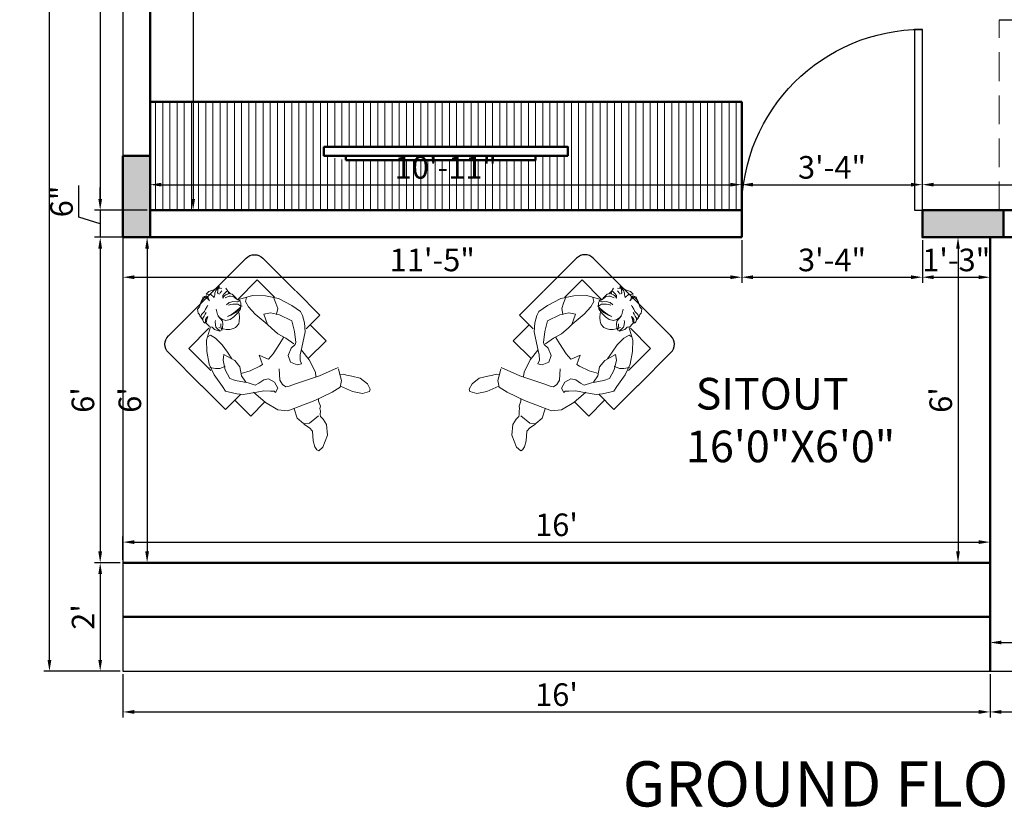
# Model space of a CAD drawing. Units: inches. Extents: x 3064 to 19385, y 846 to 15425.
# Tile 81 of 108: x 7077 to 7295, y 850 to 1024. Entities that reach past the tile are written whole.
import ezdxf

# ---------------------------------------------------------------- set-up
doc = ezdxf.new("R2010")
doc.units = ezdxf.units.IN
doc.linetypes.add('DASHED', pattern=[19.05, 12.7, -6.35])
for name, color, linetype, lineweight in [('A-ANNO-DIMS', 2, 'Continuous', 18), ('A-ANNO-TEXT', 7, 'Continuous', 25), ('A-AREA-IDEN', 3, 'Continuous', 18), ('A-COLS', 1, 'Continuous', 35), ('A-DOOR', 3, 'Continuous', 25), ('A-FLOR-STRS', 2, 'Continuous', 25), ('A-FLOR-STRS-OVHD', 2, 'DASHED', 18), ('A-FURN', 8, 'Continuous', 18), ('A-FURN-PATT', 252, 'Continuous', 13), ('A-WALL', 7, 'Continuous', 50), ('C-PROP', 6, 'Continuous', 25)]:
    doc.layers.add(name, color=color, linetype=linetype, lineweight=lineweight)
doc.layers.add('NOITHAT', color=21, linetype='Continuous')
doc.styles.get("Standard").update_dxf_attribs({"font": 'arial.ttf'})
doc.dimstyles.new('ISO-25', dxfattribs={"dimtxt": 9, "dimasz": 2.5, "dimexe": 1.25, "dimexo": 0.625, "dimtad": 1, "dimdec": 1, "dimlunit": 3, "dimtxsty": 'Standard', "dimcen": 2.5, "dimadec": 0, "dimazin": 0, "dimtfac": 1, "dimtdec": 1, "dimtmove": 0, "dimatfit": 3, "dimfxl": 1, "dimarcsym": 0})

# ---------------------------------------------------------------- blocks, each defined once
blk = doc.blocks.new('*U2')
for p, q in [((0, 0), (0, -6)), ((40, 0), (40, -6))]:
    blk.add_line(p, q)
blk.add_lwpolyline([(0, 0), (0, 40), (1.75, 40), (1.75, 0)], close=True)
blk.add_arc((0, 0), 40, 0, 90)
blk = doc.blocks.new('*D299')
at = {"layer": 'A-ANNO-DIMS', "color": 0, "lineweight": -2, "transparency": 16777216}
for p, q in [((7099.08, 1252.34), (7093.43, 1252.34)), ((7094.68, 1249.84), (7094.68, 984.84)), ((7105.08, 982.34), (7093.43, 982.34))]:
    blk.add_line(p, q, dxfattribs=at)
at = {"layer": 'A-ANNO-DIMS', "color": 0, "transparency": 16777216}
for points in [[(7094.26, 1249.84), (7095.09, 1249.84), (7094.68, 1252.34)], [(7094.26, 984.84), (7095.09, 984.84), (7094.68, 982.34)]]:
    blk.add_solid(points, dxfattribs=at)
at = {"layer": 'Defpoints', "color": 0, "transparency": 16777216}
for p in [(7099.71, 1252.34), (7094.68, 982.34), (7105.71, 982.34)]:
    blk.add_point(p, dxfattribs=at)
at = {"layer": 'A-ANNO-DIMS', "color": 0, "transparency": 16777216, "insert": (7091.5, 1117.34), "char_height": 5, "attachment_point": 5, "rotation": 90}
blk.add_mtext('22\'-6"', dxfattribs=at)
blk = doc.blocks.new('*D300')
at = {"layer": 'A-ANNO-DIMS', "color": 0, "lineweight": -2, "transparency": 16777216}
for p, q in [((7089.94, 980.76), (7089.94, 987.79)), ((7094.68, 984.84), (7094.68, 987.34)), ((7105.08, 982.34), (7093.43, 982.34)), ((7094.68, 982.34), (7094.68, 976.34)), ((7094.68, 982.34), (7094.68, 976.34)), ((7094.68, 979.34), (7089.94, 980.76)), ((7105.08, 976.34), (7093.43, 976.34)), ((7094.68, 973.84), (7094.68, 971.34))]:
    blk.add_line(p, q, dxfattribs=at)
at = {"layer": 'A-ANNO-DIMS', "color": 0, "transparency": 16777216}
for points in [[(7094.26, 984.84), (7095.09, 984.84), (7094.68, 982.34)], [(7094.26, 973.84), (7095.09, 973.84), (7094.68, 976.34)]]:
    blk.add_solid(points, dxfattribs=at)
at = {"layer": 'Defpoints', "color": 0, "transparency": 16777216}
for p in [(7105.71, 982.34), (7094.68, 976.34), (7105.71, 976.34)]:
    blk.add_point(p, dxfattribs=at)
at = {"layer": 'A-ANNO-DIMS', "color": 0, "transparency": 16777216, "insert": (7086.76, 984.27), "char_height": 5, "attachment_point": 5, "rotation": 90}
blk.add_mtext('6"', dxfattribs=at)
blk = doc.blocks.new('*D301')
at = {"layer": 'A-ANNO-DIMS', "color": 0, "lineweight": -2, "transparency": 16777216}
for p, q in [((7105.08, 976.34), (7093.43, 976.34)), ((7094.68, 973.84), (7094.68, 906.84)), ((7099.08, 904.34), (7093.43, 904.34))]:
    blk.add_line(p, q, dxfattribs=at)
at = {"layer": 'A-ANNO-DIMS', "color": 0, "transparency": 16777216}
for points in [[(7094.26, 973.84), (7095.09, 973.84), (7094.68, 976.34)], [(7094.26, 906.84), (7095.09, 906.84), (7094.68, 904.34)]]:
    blk.add_solid(points, dxfattribs=at)
at = {"layer": 'Defpoints', "color": 0, "transparency": 16777216}
for p in [(7105.71, 976.34), (7094.68, 904.34), (7099.71, 904.34)]:
    blk.add_point(p, dxfattribs=at)
at = {"layer": 'A-ANNO-DIMS', "color": 0, "transparency": 16777216, "insert": (7091.5, 940.34), "char_height": 5, "attachment_point": 5, "rotation": 90}
blk.add_mtext("6'", dxfattribs=at)
blk = doc.blocks.new('*D302')
at = {"layer": 'A-ANNO-DIMS', "color": 0, "lineweight": -2, "transparency": 16777216}
for p, q in [((7099.08, 904.34), (7093.43, 904.34)), ((7094.68, 901.84), (7094.68, 882.84)), ((7099.08, 880.34), (7093.43, 880.34))]:
    blk.add_line(p, q, dxfattribs=at)
at = {"layer": 'A-ANNO-DIMS', "color": 0, "transparency": 16777216}
for points in [[(7094.26, 901.84), (7095.09, 901.84), (7094.68, 904.34)], [(7094.26, 882.84), (7095.09, 882.84), (7094.68, 880.34)]]:
    blk.add_solid(points, dxfattribs=at)
at = {"layer": 'Defpoints', "color": 0, "transparency": 16777216}
for p in [(7099.71, 904.34), (7094.68, 880.34), (7099.71, 880.34)]:
    blk.add_point(p, dxfattribs=at)
at = {"layer": 'A-ANNO-DIMS', "color": 0, "transparency": 16777216, "insert": (7091.54, 892.34), "char_height": 5, "attachment_point": 5, "rotation": 90}
blk.add_mtext("2'", dxfattribs=at)
blk = doc.blocks.new('*D303')
at = {"layer": 'A-ANNO-DIMS', "color": 0, "lineweight": -2, "transparency": 16777216}
for p, q in [((7099.08, 1396.34), (7082.19, 1396.34)), ((7083.44, 882.84), (7083.44, 1393.84)), ((7099.08, 880.34), (7082.19, 880.34))]:
    blk.add_line(p, q, dxfattribs=at)
at = {"layer": 'A-ANNO-DIMS', "color": 0, "transparency": 16777216}
for points in [[(7083.02, 1393.84), (7083.86, 1393.84), (7083.44, 1396.34)], [(7083.02, 882.84), (7083.86, 882.84), (7083.44, 880.34)]]:
    blk.add_solid(points, dxfattribs=at)
at = {"layer": 'Defpoints', "color": 0, "transparency": 16777216}
for p in [(7083.44, 1396.34), (7099.71, 1396.34), (7099.71, 880.34)]:
    blk.add_point(p, dxfattribs=at)
at = {"layer": 'A-ANNO-DIMS', "color": 0, "transparency": 16777216, "insert": (7080.26, 1138.34), "char_height": 5, "attachment_point": 5, "rotation": 90}
blk.add_mtext("43'", dxfattribs=at)
blk = doc.blocks.new('*D304')
at = {"layer": 'A-ANNO-DIMS', "color": 0, "lineweight": -2, "transparency": 16777216}
for p, q in [((7099.71, 879.71), (7099.71, 870.08)), ((7291.71, 879.71), (7291.71, 870.08)), ((7102.21, 871.33), (7289.21, 871.33))]:
    blk.add_line(p, q, dxfattribs=at)
at = {"layer": 'A-ANNO-DIMS', "color": 0, "transparency": 16777216}
for points in [[(7102.21, 871.75), (7102.21, 870.91), (7099.71, 871.33)], [(7289.21, 871.75), (7289.21, 870.91), (7291.71, 871.33)]]:
    blk.add_solid(points, dxfattribs=at)
at = {"layer": 'Defpoints', "color": 0, "transparency": 16777216}
for p in [(7099.71, 880.34), (7291.71, 880.34), (7291.71, 871.33)]:
    blk.add_point(p, dxfattribs=at)
at = {"layer": 'A-ANNO-DIMS', "color": 0, "transparency": 16777216, "insert": (7195.71, 874.51), "char_height": 5, "attachment_point": 5}
blk.add_mtext("16'", dxfattribs=at)
blk = doc.blocks.new('*D305')
at = {"layer": 'A-ANNO-DIMS', "color": 0, "lineweight": -2, "transparency": 16777216}
for p, q in [((7291.71, 879.71), (7291.71, 870.08)), ((7441.71, 879.71), (7441.71, 870.08)), ((7294.21, 871.33), (7439.21, 871.33))]:
    blk.add_line(p, q, dxfattribs=at)
at = {"layer": 'A-ANNO-DIMS', "color": 0, "transparency": 16777216}
for points in [[(7294.21, 871.75), (7294.21, 870.91), (7291.71, 871.33)], [(7439.21, 871.75), (7439.21, 870.91), (7441.71, 871.33)]]:
    blk.add_solid(points, dxfattribs=at)
at = {"layer": 'Defpoints', "color": 0, "transparency": 16777216}
for p in [(7291.71, 880.34), (7441.71, 880.34), (7441.71, 871.33)]:
    blk.add_point(p, dxfattribs=at)
at = {"layer": 'A-ANNO-DIMS', "color": 0, "transparency": 16777216, "insert": (7366.71, 874.51), "char_height": 5, "attachment_point": 5}
blk.add_mtext('12\'-6"', dxfattribs=at)
blk = doc.blocks.new('*D223')
at = {"layer": 'A-ANNO-DIMS', "color": 0, "lineweight": -2, "transparency": 16777216}
for p, q in [((7106.33, 1252.34), (7116.51, 1252.34)), ((7115.26, 1249.84), (7115.26, 984.84)), ((7106.33, 982.34), (7116.51, 982.34))]:
    blk.add_line(p, q, dxfattribs=at)
at = {"layer": 'A-ANNO-DIMS', "color": 0, "transparency": 16777216}
for points in [[(7114.84, 1249.84), (7115.67, 1249.84), (7115.26, 1252.34)], [(7114.84, 984.84), (7115.67, 984.84), (7115.26, 982.34)]]:
    blk.add_solid(points, dxfattribs=at)
at = {"layer": 'Defpoints', "color": 0, "transparency": 16777216}
for p in [(7105.71, 1252.34), (7105.71, 982.34), (7115.26, 982.34)]:
    blk.add_point(p, dxfattribs=at)
at = {"layer": 'A-ANNO-DIMS', "color": 0, "transparency": 16777216, "insert": (7112.08, 1117.34), "char_height": 5, "attachment_point": 5, "rotation": 90}
blk.add_mtext('22\'-6"', dxfattribs=at)
blk = doc.blocks.new('*D272')
at = {"layer": 'A-ANNO-DIMS', "color": 0, "lineweight": -2, "transparency": 16777216}
for p, q in [((7105.71, 982.96), (7105.71, 989.23)), ((7108.21, 987.98), (7234.21, 987.98)), ((7236.71, 982.96), (7236.71, 989.23))]:
    blk.add_line(p, q, dxfattribs=at)
at = {"layer": 'A-ANNO-DIMS', "color": 0, "transparency": 16777216}
for points in [[(7108.21, 988.4), (7108.21, 987.57), (7105.71, 987.98)], [(7234.21, 988.4), (7234.21, 987.57), (7236.71, 987.98)]]:
    blk.add_solid(points, dxfattribs=at)
at = {"layer": 'Defpoints', "color": 0, "transparency": 16777216}
for p in [(7236.71, 987.98), (7105.71, 982.34), (7236.71, 982.34)]:
    blk.add_point(p, dxfattribs=at)
at = {"layer": 'A-ANNO-DIMS', "color": 0, "transparency": 16777216, "insert": (7171.21, 991.16), "char_height": 5, "attachment_point": 5}
blk.add_mtext('10\'-11"', dxfattribs=at)
blk = doc.blocks.new('*D273')
at = {"layer": 'A-ANNO-DIMS', "color": 0, "lineweight": -2, "transparency": 16777216}
for p, q in [((7236.71, 982.96), (7236.71, 989.23)), ((7239.21, 987.98), (7274.21, 987.98)), ((7276.71, 982.96), (7276.71, 989.23))]:
    blk.add_line(p, q, dxfattribs=at)
at = {"layer": 'A-ANNO-DIMS', "color": 0, "transparency": 16777216}
for points in [[(7239.21, 988.4), (7239.21, 987.57), (7236.71, 987.98)], [(7274.21, 988.4), (7274.21, 987.57), (7276.71, 987.98)]]:
    blk.add_solid(points, dxfattribs=at)
at = {"layer": 'Defpoints', "color": 0, "transparency": 16777216}
for p in [(7276.71, 987.98), (7236.71, 982.34), (7276.71, 982.34)]:
    blk.add_point(p, dxfattribs=at)
at = {"layer": 'A-ANNO-DIMS', "color": 0, "transparency": 16777216, "insert": (7256.71, 991.16), "char_height": 5, "attachment_point": 5}
blk.add_mtext('3\'-4"', dxfattribs=at)
blk = doc.blocks.new('*D274')
at = {"layer": 'A-ANNO-DIMS', "color": 0, "lineweight": -2, "transparency": 16777216}
for p, q in [((7276.71, 982.96), (7276.71, 989.23)), ((7279.21, 987.98), (7433.21, 987.98)), ((7435.71, 982.96), (7435.71, 989.23))]:
    blk.add_line(p, q, dxfattribs=at)
at = {"layer": 'A-ANNO-DIMS', "color": 0, "transparency": 16777216}
for points in [[(7279.21, 988.4), (7279.21, 987.57), (7276.71, 987.98)], [(7433.21, 988.4), (7433.21, 987.57), (7435.71, 987.98)]]:
    blk.add_solid(points, dxfattribs=at)
at = {"layer": 'Defpoints', "color": 0, "transparency": 16777216}
for p in [(7435.71, 987.98), (7276.71, 982.34), (7435.71, 982.34)]:
    blk.add_point(p, dxfattribs=at)
at = {"layer": 'A-ANNO-DIMS', "color": 0, "transparency": 16777216, "insert": (7356.21, 991.16), "char_height": 5, "attachment_point": 5}
blk.add_mtext('13\'-3"', dxfattribs=at)
blk = doc.blocks.new('*D240')
at = {"layer": 'A-ANNO-DIMS', "color": 0, "lineweight": -2, "transparency": 16777216}
for p, q in [((7100.33, 976.34), (7106.32, 976.34)), ((7105.07, 973.84), (7105.07, 906.84)), ((7100.33, 904.34), (7106.32, 904.34))]:
    blk.add_line(p, q, dxfattribs=at)
at = {"layer": 'A-ANNO-DIMS', "color": 0, "transparency": 16777216}
for points in [[(7104.65, 973.84), (7105.48, 973.84), (7105.07, 976.34)], [(7104.65, 906.84), (7105.48, 906.84), (7105.07, 904.34)]]:
    blk.add_solid(points, dxfattribs=at)
at = {"layer": 'Defpoints', "color": 0, "transparency": 16777216}
for p in [(7099.71, 976.34), (7099.71, 904.34), (7105.07, 904.34)]:
    blk.add_point(p, dxfattribs=at)
at = {"layer": 'A-ANNO-DIMS', "color": 0, "transparency": 16777216, "insert": (7101.89, 940.34), "char_height": 5, "attachment_point": 5, "rotation": 90}
blk.add_mtext("6'", dxfattribs=at)
blk = doc.blocks.new('*D241')
at = {"layer": 'A-ANNO-DIMS', "color": 0, "lineweight": -2, "transparency": 16777216}
for p, q in [((7099.71, 975.71), (7099.71, 966.25)), ((7236.71, 975.71), (7236.71, 966.25)), ((7102.21, 967.5), (7234.21, 967.5))]:
    blk.add_line(p, q, dxfattribs=at)
at = {"layer": 'A-ANNO-DIMS', "color": 0, "transparency": 16777216}
for points in [[(7102.21, 967.92), (7102.21, 967.09), (7099.71, 967.5)], [(7234.21, 967.92), (7234.21, 967.09), (7236.71, 967.5)]]:
    blk.add_solid(points, dxfattribs=at)
at = {"layer": 'Defpoints', "color": 0, "transparency": 16777216}
for p in [(7099.71, 976.34), (7236.71, 976.34), (7236.71, 967.5)]:
    blk.add_point(p, dxfattribs=at)
at = {"layer": 'A-ANNO-DIMS', "color": 0, "transparency": 16777216, "insert": (7168.21, 970.68), "char_height": 5, "attachment_point": 5}
blk.add_mtext('11\'-5"', dxfattribs=at)
blk = doc.blocks.new('*D267')
at = {"layer": 'A-ANNO-DIMS', "color": 0, "lineweight": -2, "transparency": 16777216}
for p, q in [((7236.71, 975.71), (7236.71, 966.25)), ((7276.71, 975.71), (7276.71, 966.25)), ((7239.21, 967.5), (7274.21, 967.5))]:
    blk.add_line(p, q, dxfattribs=at)
at = {"layer": 'A-ANNO-DIMS', "color": 0, "transparency": 16777216}
for points in [[(7239.21, 967.92), (7239.21, 967.09), (7236.71, 967.5)], [(7274.21, 967.92), (7274.21, 967.09), (7276.71, 967.5)]]:
    blk.add_solid(points, dxfattribs=at)
at = {"layer": 'Defpoints', "color": 0, "transparency": 16777216}
for p in [(7236.71, 976.34), (7276.71, 976.34), (7276.71, 967.5)]:
    blk.add_point(p, dxfattribs=at)
at = {"layer": 'A-ANNO-DIMS', "color": 0, "transparency": 16777216, "insert": (7256.71, 970.68), "char_height": 5, "attachment_point": 5}
blk.add_mtext('3\'-4"', dxfattribs=at)
blk = doc.blocks.new('*D268')
at = {"layer": 'A-ANNO-DIMS', "color": 0, "lineweight": -2, "transparency": 16777216}
for p, q in [((7276.71, 975.71), (7276.71, 966.25)), ((7291.71, 975.71), (7291.71, 966.25)), ((7279.21, 967.5), (7289.21, 967.5))]:
    blk.add_line(p, q, dxfattribs=at)
at = {"layer": 'A-ANNO-DIMS', "color": 0, "transparency": 16777216}
for points in [[(7279.21, 967.92), (7279.21, 967.09), (7276.71, 967.5)], [(7289.21, 967.92), (7289.21, 967.09), (7291.71, 967.5)]]:
    blk.add_solid(points, dxfattribs=at)
at = {"layer": 'Defpoints', "color": 0, "transparency": 16777216}
for p in [(7276.71, 976.34), (7291.71, 976.34), (7291.71, 967.5)]:
    blk.add_point(p, dxfattribs=at)
at = {"layer": 'A-ANNO-DIMS', "color": 0, "transparency": 16777216, "insert": (7284.21, 970.68), "char_height": 5, "attachment_point": 5}
blk.add_mtext('1\'-3"', dxfattribs=at)
blk = doc.blocks.new('*D269')
at = {"layer": 'A-ANNO-DIMS', "color": 0, "lineweight": -2, "transparency": 16777216}
for p, q in [((7099.71, 904.96), (7099.71, 910.15)), ((7291.71, 904.96), (7291.71, 910.15)), ((7102.21, 908.9), (7289.21, 908.9))]:
    blk.add_line(p, q, dxfattribs=at)
at = {"layer": 'A-ANNO-DIMS', "color": 0, "transparency": 16777216}
for points in [[(7102.21, 909.32), (7102.21, 908.49), (7099.71, 908.9)], [(7289.21, 909.32), (7289.21, 908.49), (7291.71, 908.9)]]:
    blk.add_solid(points, dxfattribs=at)
at = {"layer": 'Defpoints', "color": 0, "transparency": 16777216}
for p in [(7291.71, 908.9), (7099.71, 904.34), (7291.71, 904.34)]:
    blk.add_point(p, dxfattribs=at)
at = {"layer": 'A-ANNO-DIMS', "color": 0, "transparency": 16777216, "insert": (7195.71, 912.08), "char_height": 5, "attachment_point": 5}
blk.add_mtext("16'", dxfattribs=at)
blk = doc.blocks.new('*D270')
at = {"layer": 'A-ANNO-DIMS', "color": 0, "lineweight": -2, "transparency": 16777216}
for p, q in [((7291.08, 976.34), (7283.35, 976.34)), ((7284.6, 973.84), (7284.6, 906.84)), ((7291.08, 904.34), (7283.35, 904.34))]:
    blk.add_line(p, q, dxfattribs=at)
at = {"layer": 'A-ANNO-DIMS', "color": 0, "transparency": 16777216}
for points in [[(7284.19, 973.84), (7285.02, 973.84), (7284.6, 976.34)], [(7284.19, 906.84), (7285.02, 906.84), (7284.6, 904.34)]]:
    blk.add_solid(points, dxfattribs=at)
at = {"layer": 'Defpoints', "color": 0, "transparency": 16777216}
for p in [(7291.71, 976.34), (7284.6, 904.34), (7291.71, 904.34)]:
    blk.add_point(p, dxfattribs=at)
at = {"layer": 'A-ANNO-DIMS', "color": 0, "transparency": 16777216, "insert": (7281.43, 940.34), "char_height": 5, "attachment_point": 5, "rotation": 90}
blk.add_mtext("6'", dxfattribs=at)
blk = doc.blocks.new('*D221')
at = {"layer": 'A-ANNO-DIMS', "color": 0, "lineweight": -2, "transparency": 16777216}
for p, q in [((7291.71, 880.96), (7291.71, 887.94)), ((7441.71, 880.96), (7441.71, 887.94)), ((7294.21, 886.69), (7439.21, 886.69))]:
    blk.add_line(p, q, dxfattribs=at)
at = {"layer": 'A-ANNO-DIMS', "color": 0, "transparency": 16777216}
for points in [[(7294.21, 887.11), (7294.21, 886.28), (7291.71, 886.69)], [(7439.21, 887.11), (7439.21, 886.28), (7441.71, 886.69)]]:
    blk.add_solid(points, dxfattribs=at)
at = {"layer": 'Defpoints', "color": 0, "transparency": 16777216}
for p in [(7441.71, 886.69), (7291.71, 880.34), (7441.71, 880.34)]:
    blk.add_point(p, dxfattribs=at)
at = {"layer": 'A-ANNO-DIMS', "color": 0, "transparency": 16777216, "insert": (7366.71, 889.87), "char_height": 5, "attachment_point": 5}
blk.add_mtext('12\'-6"', dxfattribs=at)
blk = doc.blocks.new('A$C48E80792')
for p, q in [((230.8, 792.5), (252, 804.1)), ((252, 804.1), (267.8, 807.6)), ((253.5, 801.9), (261.1, 805.7)), ((261.1, 805.7), (274.4, 805.7)), ((267.8, 807.6), (270.5, 811.7)), ((284, 805.7), (270.6, 811.4)), ((274.4, 805.7), (278.3, 805.7)), ((278.3, 805.7), (278.3, 798.1)), ((278.3, 798.1), (280.2, 788.5)), ((284, 794.3), (284, 805.7)), ((289.7, 811.4), (305.5, 811.7)), ((289.7, 811.4), (303, 796.2)), ((305.5, 811.7), (317.9, 805.5)), ((317.9, 805.5), (328.1, 800)), ((328.1, 800), (343.9, 798)), ((343.9, 798), (352.1, 795.9)), ((202, 746.6), (204.7, 764.4)), ((202, 746.6), (205.8, 759.9)), ((204.7, 764.4), (207.4, 769.9)), ((205.8, 759.9), (213.4, 763.8)), ((207.4, 769.9), (208.1, 777.4)), ((208.1, 777.4), (217.7, 791.8)), ((213.4, 763.8), (222.9, 763.8)), ((217.7, 791.8), (230.8, 792.5)), ((222.9, 763.8), (232.5, 763.8)), ((226.8, 754.2), (234.4, 756.1)), ((232.5, 763.8), (236.3, 765.7)), ((236.3, 765.7), (242, 767.6)), ((242, 767.6), (255.4, 771.4)), ((255.4, 771.4), (261.1, 773.3)), ((280.2, 786.6), (284, 794.3)), ((280.2, 788.5), (280.2, 780.9)), ((280.2, 780.9), (280.2, 786.6)), ((303, 796.2), (303, 779)), ((303, 777.1), (312.6, 782.8)), ((303, 779), (303, 777.1)), ((312.6, 782.8), (318.3, 788.5)), ((318.3, 788.5), (329.8, 792.4)), ((335.5, 786.6), (327.8, 780.9)), ((327.8, 780.9), (327.8, 775.2)), ((327.8, 748.5), (335.5, 756.1)), ((329.8, 792.4), (343.1, 794.3)), ((329.8, 771.4), (335.5, 773.3)), ((343.1, 792.4), (335.5, 786.6)), ((335.5, 773.3), (346.9, 773.3)), ((335.5, 756.1), (346.9, 758)), ((343.1, 794.3), (352.6, 794.3)), ((352.6, 792.4), (343.1, 792.4)), ((343.9, 790.4), (354.9, 782.2)), ((346.9, 758), (358.4, 758)), ((358.4, 758), (362.2, 756.1)), ((366, 769.5), (362.2, 750.4)), ((362.2, 756.1), (364.1, 750.4)), ((198.1, 735.2), (202, 742.8)), ((198.1, 727.5), (198.1, 735.2)), ((202, 727.5), (200.1, 725.6)), ((202, 742.8), (207.7, 748.5)), ((211.5, 737.1), (202, 727.5)), ((202, 723.7), (209.6, 729.4)), ((202, 716.1), (202, 723.7)), ((202, 706.6), (202, 716.1)), ((207.7, 748.5), (217.2, 750.4)), ((209.6, 729.4), (219.1, 735.2)), ((219.1, 739), (211.5, 737.1)), ((217.2, 750.4), (226.8, 754.2)), ((226.8, 739), (219.1, 739)), ((219.1, 735.2), (226.8, 739)), ((226.8, 739), (226.8, 739)), ((261.6, 715.7), (260.3, 708.9)), ((274, 735.6), (261.6, 715.7)), ((318.3, 718), (333.6, 716.1)), ((329.8, 748.5), (327.8, 748.5)), ((335.5, 750.4), (329.8, 748.5)), ((333.6, 716.1), (339.3, 712.3)), ((337.4, 750.4), (335.5, 750.4)), ((352.6, 735.2), (335.5, 742.8)), ((341.2, 750.4), (337.4, 750.4)), ((346.9, 750.4), (341.2, 750.4)), ((354.5, 746.6), (346.9, 750.4)), ((356.5, 731.3), (352.6, 735.2)), ((362.2, 742.8), (354.5, 746.6)), ((362.2, 750.4), (356.5, 746.6)), ((362.2, 723.7), (356.5, 731.3)), ((367.9, 733.3), (362.2, 742.8)), ((364.1, 718), (362.2, 723.7)), ((364.1, 750.4), (364.1, 742.8)), ((364.1, 742.8), (364.1, 739)), ((366, 706.6), (364.1, 718)), ((367.9, 706.6), (367.9, 733.3)), ((151.7, 671.2), (119.2, 637.1)), ((204, 699.4), (151.7, 671.2)), ((165.1, 679.5), (178.4, 675)), ((178.4, 675), (185.1, 650.5)), ((202, 702.8), (202, 706.6)), ((207.7, 693.2), (202, 702.8)), ((207.7, 679.9), (207.7, 693.2)), ((219.1, 658.9), (207.7, 679.9)), ((219.1, 681.8), (224.8, 691.3)), ((219.1, 670.3), (219.1, 681.8)), ((224.8, 691.3), (232.5, 700.8)), ((227.3, 673.2), (235.6, 655.4)), ((232.5, 700.8), (238.2, 704.7)), ((236.3, 670.3), (243.9, 678)), ((257.3, 679.9), (249.6, 670.3)), ((259.2, 708.5), (257.3, 679.9)), ((260.3, 708.9), (259.6, 699.3)), ((259.6, 699.3), (261.6, 685.6)), ((261.6, 685.6), (269.2, 671.8)), ((269.2, 671.8), (285.6, 662.9)), ((302.1, 672.5), (287, 679.4)), ((287, 679.4), (304.8, 673.9)), ((323.3, 667), (302.1, 672.5)), ((304.8, 673.9), (323.3, 670.5)), ((331.7, 706.6), (324, 710.4)), ((339.3, 700.8), (331.7, 706.6)), ((339.3, 712.3), (346.9, 708.5)), ((346.9, 693.2), (339.3, 700.8)), ((346.9, 708.5), (358.4, 695.1)), ((354.5, 685.6), (346.9, 693.2)), ((356.5, 676.1), (354.5, 685.6)), ((356.3, 668.4), (367.2, 680.1)), ((362.2, 666.5), (356.5, 676.1)), ((358.4, 695.1), (360.3, 693.2)), ((360.3, 693.2), (366, 691.3)), ((367.9, 698.9), (366, 706.6)), ((366, 691.3), (369.8, 689.4)), ((366.5, 698.9), (425.1, 668)), ((367.2, 680.1), (370.7, 689)), ((371.7, 691.3), (367.9, 698.9)), ((369.8, 689.4), (371.7, 689.4)), ((371.7, 689.4), (371.7, 691.3)), ((371.7, 689.4), (371.7, 689.4)), ((385.6, 670.5), (378.9, 646.1)), ((401.2, 679.5), (385.6, 670.5)), ((119.2, 637.1), (88.2, 591.5)), ((185.1, 650.5), (185.1, 610.4)), ((221, 657), (219.1, 670.3)), ((226.8, 655.1), (232.5, 664.6)), ((232.5, 657), (226.8, 655.1)), ((232.5, 664.6), (236.3, 670.3)), ((238.2, 660.8), (232.5, 657)), ((235.6, 655.4), (243.8, 644.4)), ((249.6, 670.3), (238.2, 660.8)), ((243.8, 644.4), (254.8, 633.5)), ((254.8, 633.5), (267.8, 625.9)), ((285.6, 662.9), (304.8, 659.5)), ((298, 623.9), (307.6, 630.7)), ((304.8, 659.5), (326.8, 659.5)), ((307.6, 630.7), (319.2, 640.3)), ((319.2, 640.3), (330.9, 654)), ((323.3, 670.5), (345.3, 668.4)), ((337.7, 666.4), (323.3, 667)), ((326.8, 659.5), (340.5, 661.6)), ((330.9, 654), (334, 660.6)), ((356.3, 669.8), (337.7, 666.4)), ((340.5, 661.6), (348.7, 664.3)), ((345.3, 668.4), (356.3, 668.4)), ((348.7, 664.3), (352.1, 667.7)), ((352.1, 667.7), (356.3, 669.8)), ((356.3, 668.4), (358.3, 669.8)), ((378.9, 646.1), (376.7, 603.8)), ((425.1, 668), (462.5, 627.3)), ((88.2, 591.5), (70.3, 544.3)), ((185.1, 610.4), (178.4, 572.6)), ((267.8, 625.9), (276.7, 622.5)), ((276.7, 622.5), (283.6, 621.8)), ((283.6, 621.8), (298, 623.9)), ((376.7, 603.8), (383.3, 537)), ((462.5, 627.3), (493.4, 580.1)), ((485.8, 606), (472.4, 574.8)), ((80.4, 579.3), (93.8, 559.2)), ((93.8, 559.2), (107.1, 545.9)), ((107.1, 545.9), (125, 539.2)), ((119.2, 526.5), (141.9, 562.2)), ((141.9, 562.2), (161.5, 576.9)), ((161.5, 576.9), (175.7, 525.7)), ((178.4, 572.6), (171.7, 539.2)), ((402.3, 576.9), (383.3, 535)), ((426.7, 560.6), (402.3, 576.9)), ((447.9, 528.1), (426.7, 560.6)), ((461.3, 552.6), (441.3, 539.2)), ((472.4, 574.8), (461.3, 552.6)), ((493.4, 580.1), (513, 518.3)), ((70.3, 544.3), (60.6, 484.2)), ((106.8, 485.6), (119.2, 526.5)), ((125, 539.2), (129.4, 537)), ((175.7, 525.7), (172, 490.5)), ((383.3, 535), (383.3, 512.7)), ((383.3, 512.7), (385.2, 475.7)), ((441.3, 539.2), (441.3, 537)), ((467.4, 472.8), (447.9, 528.1)), ((513, 518.3), (521.1, 474.4)), ((60.6, 484.2), (55.7, 461.4)), ((55.7, 461.4), (62.2, 451.6)), ((117.5, 463), (106.8, 485.6)), ((149.1, 418.9), (117.5, 463)), ((172, 490.5), (149.7, 459)), ((156.1, 468), (191.8, 447.9)), ((247.5, 430.1), (265.3, 468)), ((265.3, 468), (276.4, 439)), ((385.2, 475.7), (396.3, 438.6)), ((443, 432.1), (467.4, 472.8)), ((521.1, 474.4), (514.6, 456.5)), ((62.2, 451.6), (81.7, 419.1)), ((81.7, 419.1), (99.6, 398)), ((149.7, 459), (143.7, 426.5)), ((191.8, 447.9), (234.1, 432.3)), ((234.1, 432.3), (247.5, 430.1)), ((276.4, 439), (280.9, 427.9)), ((280.9, 427.9), (312.1, 430.1)), ((312.1, 430.1), (363.3, 441.2)), ((363.3, 441.2), (392.3, 447.9)), ((396.3, 438.6), (403.7, 397.8)), ((413.7, 396.3), (443, 432.1)), ((499.9, 428.9), (473.9, 399.6)), ((514.6, 456.5), (499.9, 428.9)), ((99.6, 398), (147.5, 363.6)), ((163.7, 389.7), (149.1, 418.9)), ((180, 384.8), (163.7, 389.7)), ((204.4, 379.9), (180, 384.8)), ((222.3, 368.5), (204.4, 379.9)), ((338.8, 352.4), (351.9, 380.1)), ((351.9, 380.1), (382.8, 393.1)), ((382.8, 393.1), (405.6, 391.5)), ((405.6, 391.5), (413.7, 396.3)), ((473.9, 399.6), (433.2, 373.6)), ((136.8, 373.8), (142.3, 307)), ((147.5, 363.6), (171.9, 347.4)), ((171.9, 347.4), (191.4, 326.2)), ((230.5, 340.9), (222.3, 368.5)), ((222.3, 313.2), (230.5, 340.9)), ((285.1, 367.1), (252.6, 331.3)), ((350.2, 324.8), (338.8, 352.4)), ((389.3, 345.9), (373, 329.7)), ((405.6, 355.7), (389.3, 345.9)), ((407.4, 355.2), (401.9, 303.3)), ((433.2, 373.6), (405.6, 355.7)), ((142.3, 307), (157.1, 247.7)), ((191.4, 326.2), (202.8, 314.8)), ((202.8, 314.8), (202.8, 306.7)), ((202.8, 306.7), (222.3, 313.2)), ((252.6, 331.3), (247.7, 310.1)), ((247.7, 310.1), (251, 292.3)), ((366.5, 315), (350.2, 324.8)), ((373, 329.7), (366.5, 315)), ((401.9, 303.3), (383.3, 247.7)), ((251, 292.3), (262.4, 284.1)), ((262.4, 284.1), (288.4, 272.7)), ((288.4, 272.7), (332.3, 250)), ((157.1, 247.7), (185, 214.4)), ((185, 214.4), (249.8, 184.7)), ((332.3, 250), (384.4, 223.9)), ((383.3, 247.7), (372.2, 232.9)), ((384.4, 223.9), (466, 193.4)), ((209.1, 201.4), (190.5, 164.4)), ((249.8, 184.7), (296.2, 164.4)), ((437.1, 144), (452.7, 171.9)), ((452.7, 171.9), (462.5, 188.2)), ((190.5, 164.4), (194.2, 129.2)), ((192.4, 126.7), (199, 98.4)), ((194.2, 129.2), (212.8, 112.5)), ((287.5, 125.1), (295.8, 130.1)), ((295.8, 130.1), (305.5, 151.4)), ((296.2, 164.4), (374.1, 136.6)), ((305.5, 151.4), (311, 157)), ((374.1, 136.6), (413, 127.3)), ((413, 127.3), (437.1, 144)), ((417.2, 129.7), (436.8, 77.9)), ((461.2, 158.8), (450.1, 164.4)), ((468.1, 144.2), (461.2, 158.8)), ((480.4, 126.2), (468.1, 144.2)), ((500.2, 94.8), (480.4, 126.2)), ((199, 98.4), (197.4, 78.4)), ((212.8, 112.5), (261.8, 106.9)), ((265.8, 98.4), (270.8, 106.7)), ((265.8, 91.7), (265.8, 98.4)), ((265.8, 83.4), (265.8, 91.7)), ((270.8, 106.7), (280.8, 115.1)), ((280.8, 115.1), (287.5, 125.1)), ((505.1, 56.7), (500.2, 94.8)), ((170.7, 48.4), (157.3, 25)), ((197.4, 78.4), (170.7, 48.4)), ((230.7, 21.7), (259.1, 56.7)), ((259.1, 56.7), (265.8, 83.4)), ((436.8, 77.9), (461.5, 41.9)), ((496.7, 31.6), (505.1, 56.7)), ((157.3, 25), (154, 10)), ((154, 10), (157.3, 1.7)), ((157.3, 1.7), (180.7, 0)), ((180.7, 0), (230.7, 21.7)), ((461.5, 41.9), (488.5, 26.9)), ((488.5, 26.9), (496.7, 31.6))]:
    blk.add_line(p, q)
blk.add_arc((337.3, 639.4), 150, 89.3152, 90)
at = {"layer": 'NOITHAT'}
for p, q in [((0.2, 550.4), (0, 405.9)), ((569, 405.9), (569.1, 549.9))]:
    blk.add_line(p, q, dxfattribs=at)
blk.add_lwpolyline([(0.1, 548.9), (0.1, 748.9, -0.414214), (50.1, 798.9), (518.1, 798.9, -0.414214), (568.1, 748.9), (568.1, 551.9)], format="xyb", dxfattribs=at)
for points in [[(195.1, 699.9), (74.1, 699.9), (74.1, 567.9)], [(486.1, 596.9), (486.1, 699.9), (369.1, 699.9)], [(92.1, 405.9), (0, 405.9)], [(56.1, 405.9), (56.1, 309.9), (142.1, 309.9)], [(402.6, 309.9), (510.1, 309.9), (510.1, 405.9)], [(486.1, 405.9), (569, 405.9)]]:
    blk.add_lwpolyline(points, dxfattribs=at)

msp = doc.modelspace()

# ---------------------------------------------------------------- hatches: boundary and pattern name
at = {"layer": 'A-COLS'}
h = msp.add_hatch(color=256, dxfattribs=at)
h.dxf.hatch_style = 1
h.paths.add_polyline_path([(7099.71, 976.34), (7105.71, 976.34), (7105.71, 994.34), (7099.71, 994.34)])
h = msp.add_hatch(color=256, dxfattribs=at)
h.dxf.hatch_style = 1
h.paths.add_polyline_path([(7294.71, 976.34), (7294.71, 982.34), (7276.71, 982.34), (7276.71, 976.34)])
at = {"layer": 'A-FURN-PATT'}
h = msp.add_hatch(dxfattribs=at)
h.set_pattern_fill('ANSI31', color=256, scale=0.5, angle=45)
h.set_pattern_definition([(90, (1784.0376, -1e-11), (-1.5875, 0), [])])
h.paths.add_polyline_path([(7236.71, 982.34), (7236.71, 1006.34), (7105.71, 1006.34), (7105.71, 982.34)])
h.paths.add_polyline_path([(7198.21, 994.37), (7191.03, 994.37), (7191.03, 993.37), (7149.03, 993.37), (7144.21, 994.37), (7144.21, 996.37), (7198.21, 996.37)], flags=16)

# ---------------------------------------------------------------- linework, layer by layer
at = {"layer": 'A-FLOR-STRS'}
msp.add_line((7393.71, 1024.34), (7293.71, 1024.34), dxfattribs=at)
at = {"layer": 'A-FLOR-STRS-OVHD', "ltscale": 0.5}
msp.add_line((7293.71, 982.34), (7293.71, 1024.34), dxfattribs=at)
at = {"layer": 'A-WALL'}
for p, q in [((7105.71, 1390.34), (7105.71, 982.34)), ((7236.71, 1006.34), (7105.71, 1006.34)), ((7236.71, 976.34), (7236.71, 1006.34)), ((7236.71, 982.34), (7105.71, 982.34)), ((7236.71, 976.34), (7236.71, 982.34)), ((7435.71, 982.34), (7276.71, 982.34)), ((7276.71, 976.34), (7276.71, 982.34)), ((7236.71, 976.34), (7099.71, 976.34)), ((7441.71, 976.34), (7276.71, 976.34)), ((7291.71, 976.34), (7291.71, 880.34)), ((7099.71, 904.34), (7291.71, 904.34)), ((7099.71, 892.34), (7291.71, 892.34))]:
    msp.add_line(p, q, dxfattribs=at)
for points in [[(7144.21, 996.37), (7198.21, 996.37), (7198.21, 994.37), (7144.21, 994.37)], [(7105.71, 976.34), (7105.71, 994.34), (7099.71, 994.34), (7099.71, 976.34)], [(7149.03, 993.37), (7191.03, 993.37), (7191.03, 994.37), (7149.03, 994.37)], [(7294.71, 982.34), (7276.71, 982.34), (7276.71, 976.34), (7294.71, 976.34)]]:
    msp.add_lwpolyline(points, close=True, dxfattribs=at)
at = {"layer": 'C-PROP'}
for p, q in [((7099.71, 1396.34), (7099.71, 880.34)), ((7099.71, 880.34), (7441.71, 880.34))]:
    msp.add_line(p, q, dxfattribs=at)

# ---------------------------------------------------------------- block references
at = {"layer": 'A-DOOR', "xscale": -1}
msp.add_blockref('*U2', (7276.71, 982.34), dxfattribs=at)
at = {"layer": 'A-FURN', "yscale": 0.0520199143446925, "zscale": 0.0520199143446925}
for p, xscale, rotation in [((7137.33, 923.28), 0.0520199143446925, 45.00000000000001), ((7193.5, 923.28), -0.0520199143446925, 315)]:
    msp.add_blockref('A$C48E80792', p, dxfattribs=dict(at, xscale=xscale, rotation=rotation))

# ---------------------------------------------------------------- texts
at = {"layer": 'A-ANNO-TEXT', "insert": (7210.37, 860.41), "char_height": 10, "attachment_point": 1}
msp.add_mtext_dynamic_manual_height_columns('GROUND FLOOR PLAN', width=200.9739, gutter_width=12.5, heights=[0], dxfattribs=at)
at = {"layer": 'A-AREA-IDEN', "insert": (7224.37, 945.24), "char_height": 7, "attachment_point": 1}
msp.add_mtext_dynamic_manual_height_columns(' SITOUT\\P16\'0"X6\'0"', width=67.5924, gutter_width=12.5, heights=[0], dxfattribs=at)

# ---------------------------------------------------------------- dimensions: what is measured, and where the dimension line sits
at = {"layer": 'A-ANNO-DIMS'}
for base, p1, p2, override, picture, middle in [((7083.44, 1396.34), (7099.71, 880.34), (7099.71, 1396.34), {"dimtxt": 5, "dimclrd": 0, "dimclre": 0, "dimclrt": 0}, '*D303', (7080.26, 1138.34)), ((7094.68, 982.34), (7099.71, 1252.34), (7105.71, 982.34), {"dimtxt": 5, "dimclrd": 0, "dimclre": 0, "dimclrt": 0, "dimtmove": 1}, '*D299', (7091.5, 1117.34)), ((7115.26, 982.34), (7105.71, 1252.34), (7105.71, 982.34), {"dimtxt": 5, "dimclrd": 0, "dimclre": 0, "dimclrt": 0}, '*D223', (7112.08, 1117.34)), ((7094.68, 976.34), (7105.71, 982.34), (7105.71, 976.34), {"dimtxt": 5, "dimclrd": 0, "dimclre": 0, "dimclrt": 0, "dimtmove": 1}, '*D300', (7086.76, 981.39)), ((7094.68, 904.34), (7105.71, 976.34), (7099.71, 904.34), {"dimtxt": 5, "dimclrd": 0, "dimclre": 0, "dimclrt": 0, "dimtmove": 1}, '*D301', (7091.5, 940.34)), ((7105.07, 904.34), (7099.71, 976.34), (7099.71, 904.34), {"dimtxt": 5, "dimclrd": 0, "dimclre": 0, "dimclrt": 0}, '*D240', (7101.89, 940.34)), ((7284.6, 904.34), (7291.71, 976.34), (7291.71, 904.34), {"dimtxt": 5, "dimclrd": 0, "dimclre": 0, "dimclrt": 0}, '*D270', (7281.43, 940.34)), ((7094.68, 880.34), (7099.71, 904.34), (7099.71, 880.34), {"dimtxt": 5, "dimclrd": 0, "dimclre": 0, "dimclrt": 0, "dimtmove": 1}, '*D302', (7091.54, 892.34))]:
    dim = msp.add_linear_dim(base=base, p1=p1, p2=p2, angle=90, dimstyle='ISO-25', override=override, dxfattribs=at)
    dim.commit()
    dim.dimension.update_dxf_attribs({"geometry": picture, "text_midpoint": middle})
for base, p1, p2, override, picture, middle in [((7236.71, 987.98), (7105.71, 982.34), (7236.71, 982.34), {"dimtxt": 5, "dimclrd": 0, "dimclre": 0, "dimclrt": 0}, '*D272', (7171.21, 991.16)), ((7276.71, 987.98), (7236.71, 982.34), (7276.71, 982.34), {"dimtxt": 5, "dimclrd": 0, "dimclre": 0, "dimclrt": 0, "dimtmove": 1}, '*D273', (7256.71, 991.16)), ((7435.71, 987.98), (7276.71, 982.34), (7435.71, 982.34), {"dimtxt": 5, "dimclrd": 0, "dimclre": 0, "dimclrt": 0, "dimtmove": 1}, '*D274', (7356.21, 991.16)), ((7236.71, 967.5), (7099.71, 976.34), (7236.71, 976.34), {"dimtxt": 5, "dimclrd": 0, "dimclre": 0, "dimclrt": 0}, '*D241', (7168.21, 970.68)), ((7276.71, 967.5), (7236.71, 976.34), (7276.71, 976.34), {"dimtxt": 5, "dimclrd": 0, "dimclre": 0, "dimclrt": 0, "dimtmove": 1}, '*D267', (7256.71, 970.68)), ((7291.71, 967.5), (7276.71, 976.34), (7291.71, 976.34), {"dimtxt": 5, "dimclrd": 0, "dimclre": 0, "dimclrt": 0, "dimtmove": 1}, '*D268', (7284.21, 970.68)), ((7291.71, 908.9), (7099.71, 904.34), (7291.71, 904.34), {"dimtxt": 5, "dimclrd": 0, "dimclre": 0, "dimclrt": 0}, '*D269', (7195.71, 912.08)), ((7441.71, 886.69), (7291.71, 880.34), (7441.71, 880.34), {"dimtxt": 5, "dimclrd": 0, "dimclre": 0, "dimclrt": 0}, '*D221', (7366.71, 889.87)), ((7291.71, 871.33), (7099.71, 880.34), (7291.71, 880.34), {"dimtxt": 5, "dimclrd": 0, "dimclre": 0, "dimclrt": 0}, '*D304', (7195.71, 874.51)), ((7441.71, 871.33), (7291.71, 880.34), (7441.71, 880.34), {"dimtxt": 5, "dimclrd": 0, "dimclre": 0, "dimclrt": 0, "dimtmove": 1}, '*D305', (7366.71, 874.51))]:
    dim = msp.add_linear_dim(base=base, p1=p1, p2=p2, dimstyle='ISO-25', override=override, dxfattribs=at)
    dim.commit()
    dim.dimension.update_dxf_attribs({"geometry": picture, "text_midpoint": middle})

doc.saveas('drawing.dxf')
